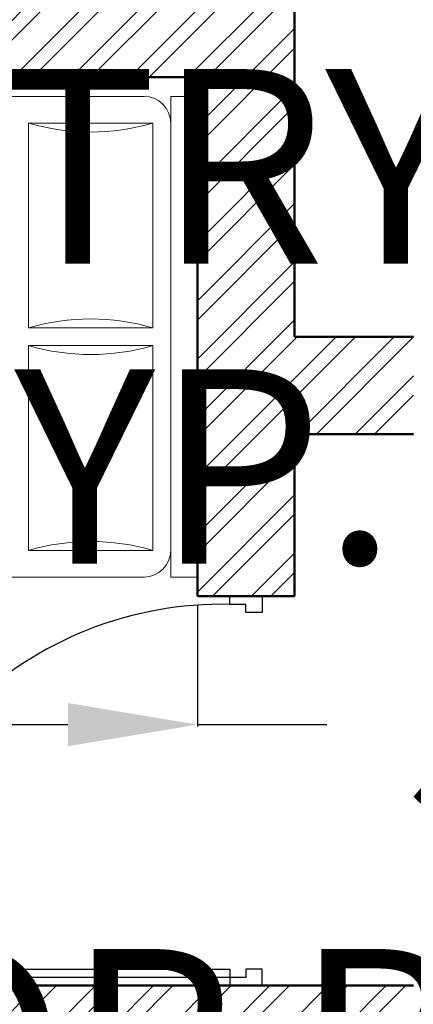
# Model space of a CAD drawing. Units: inches. Extents: x -90 to 536, y -553 to 299.
# Tile 9 of 27: x 155 to 191, y -430 to -339. Entities that reach past the tile are written whole.
import ezdxf

# ---------------------------------------------------------------- set-up
doc = ezdxf.new("R2010")
doc.units = ezdxf.units.IN
for name, color, linetype, lineweight in [('A-ANNO-DIMS', 2, 'Continuous', 18), ('A-DOOR', 4, 'Continuous', 25), ('A-WALL-PATT', 252, 'Continuous', 13), ('Furniture', 2, 'Continuous', 18), ('Outer Wall', 1, 'Continuous', 50)]:
    doc.layers.add(name, color=color, linetype=linetype, lineweight=lineweight)
doc.styles.get("Standard").update_dxf_attribs({"font": 'arial.ttf'})
doc.dimstyles.get("Standard").update_dxf_attribs({"dimtxt": 18, "dimasz": 12, "dimexe": 0.18, "dimexo": 0.0625, "dimgap": 0.09, "dimtad": 0, "dimtih": 1, "dimtoh": 1, "dimdec": 0, "dimzin": 0, "dimdsep": 46, "dimlunit": 3, "dimtxsty": 'Standard', "dimcen": 0.09, "dimadec": 0, "dimazin": 0, "dimtfac": 1, "dimtdec": 0, "dimtofl": 0, "dimtmove": 0, "dimatfit": 3, "dimfxl": 1, "dimtolj": 1, "dimtzin": 0, "dimarcsym": 0})

# ---------------------------------------------------------------- blocks, each defined once
blk = doc.blocks.new('A$C62731D1C')
for p, q in [((0.0963, 2.2932, 0.6857), (1.4679, 2.2932, 0.6857)), ((0.0963, 2.217, 0.6857), (0.0963, 2.2932, 0.6857)), ((1.4679, 2.217, 0.6857), (1.4679, 2.2932, 0.6857)), ((0.0963, 2.217, 0.6857), (1.4679, 2.217, 0.6857)), ((0.7567, 2.1662, 0.6857), (0.1725, 2.1662, 0.6857)), ((0.1725, 2.1662, 0.6857), (0.1725, 1.8106, 0.6857)), ((0.7567, 1.8106, 0.6857), (0.7567, 2.1662, 0.6857)), ((0.8075, 2.1662, 0.6857), (0.8075, 1.8106, 0.6857)), ((1.3917, 2.1662, 0.6857), (0.8075, 2.1662, 0.6857)), ((1.3917, 1.8106, 0.6857), (1.3917, 2.1662, 0.6857)), ((0.0963, 0.3882, 0.6857), (0.0963, 2.1408, 0.6857)), ((1.4679, 2.1408, 0.6857), (1.4679, 0.3882, 0.6857)), ((0.1725, 1.8106, 0.6857), (0.7567, 1.8106, 0.6857)), ((0.8075, 1.8106, 0.6857), (1.3917, 1.8106, 0.6857))]:
    blk.add_line(p, q)
for centre, radius, start, end in [((0.1725, 2.1408, 0.6857), 0.0762, 90, 180), ((1.3917, 2.1408, 0.6857), 0.0762, 0, 90), ((-0.4371, 1.9884, 0.6857), 0.635, 343.7398, 16.2602), ((1.3663, 1.9884, 0.6857), 0.635, 163.7398, 196.2602), ((0.1979, 1.9884, 0.6857), 0.635, 343.7398, 16.2602), ((2.0013, 1.9884, 0.6857), 0.635, 163.7398, 196.2602)]:
    blk.add_arc(centre, radius, start, end)
blk = doc.blocks.new('A$C0E6D7E3D')
blk.add_blockref('A$C62731D1C', (0, 0))
blk = doc.blocks.new('DOOR-36-B')
for points in [[(37.5, 36), (37.5, 34.5), (36, 34.5), (36, 35.25), (34.5, 35.25), (34.5, 36)], [(0, 0.75), (0, 1.5), (34.5, 1.5), (34.5, 0.75)], [(37.5, 0), (37.5, 1.5), (36, 1.5), (36, 0.75), (34.5, 0.75), (34.5, 0)]]:
    blk.add_lwpolyline(points, close=True)
blk.add_arc((33.758, 1.5), 33.758, 88.7408, 180)
blk = doc.blocks.new('*D27')
at = {"layer": 'A-ANNO-DIMS', "color": 0, "lineweight": -2, "transparency": 16777216}
for p, q in [((49.132, -428.616), (49.132, -434.359)), ((86.632, -428.616), (86.632, -434.359)), ((61.132, -434.179), (74.632, -434.179)), ((86.632, -434.179), (98.632, -434.179))]:
    blk.add_line(p, q, dxfattribs=at)
at = {"layer": 'A-ANNO-DIMS', "color": 0, "transparency": 16777216}
for points in [[(61.132, -432.179), (61.132, -436.179), (49.132, -434.179)], [(74.632, -432.179), (74.632, -436.179), (86.632, -434.179)]]:
    blk.add_solid(points, dxfattribs=at)
at = {"layer": 'Defpoints', "color": 0, "transparency": 16777216}
for p in [(49.132, -428.554), (86.632, -428.554), (86.632, -434.179)]:
    blk.add_point(p, dxfattribs=at)
at = {"layer": 'A-ANNO-DIMS', "color": 0, "transparency": 16777216, "insert": (195.174, -434.179), "char_height": 18, "attachment_point": 5}
blk.add_mtext('\\A1;DOOR B 38 TYP.', dxfattribs=at)
blk = doc.blocks.new('*D28')
at = {"layer": 'A-ANNO-DIMS', "color": 0, "lineweight": -2, "transparency": 16777216}
for p, q in [((92.257, -392.554), (92.257, -380.554)), ((92.257, -380.554), (104.257, -380.554)), ((86.694, -392.554), (92.437, -392.554)), ((92.257, -416.554), (92.257, -404.554)), ((86.694, -428.554), (92.437, -428.554))]:
    blk.add_line(p, q, dxfattribs=at)
at = {"layer": 'A-ANNO-DIMS', "color": 0, "transparency": 16777216}
for points in [[(90.257, -404.554), (94.257, -404.554), (92.257, -392.554)], [(90.257, -416.554), (94.257, -416.554), (92.257, -428.554)]]:
    blk.add_solid(points, dxfattribs=at)
at = {"layer": 'Defpoints', "color": 0, "transparency": 16777216}
for p in [(86.632, -392.554), (92.257, -392.554), (86.632, -428.554)]:
    blk.add_point(p, dxfattribs=at)
at = {"layer": 'A-ANNO-DIMS', "color": 0, "transparency": 16777216, "insert": (148.15, -380.554), "char_height": 18, "attachment_point": 5}
blk.add_mtext('\\A1;36 TYP.', dxfattribs=at)
blk = doc.blocks.new('*D35')
at = {"layer": 'A-ANNO-DIMS', "color": 0, "lineweight": -2, "transparency": 16777216}
for p, q in [((233.194, -331.054), (239.837, -331.054)), ((239.657, -343.054), (239.657, -343.401)), ((239.657, -362.554), (239.657, -362.207)), ((233.194, -374.554), (239.837, -374.554))]:
    blk.add_line(p, q, dxfattribs=at)
at = {"layer": 'A-ANNO-DIMS', "color": 0, "transparency": 16777216}
for points in [[(237.657, -343.054), (241.657, -343.054), (239.657, -331.054)], [(237.657, -362.554), (241.657, -362.554), (239.657, -374.554)]]:
    blk.add_solid(points, dxfattribs=at)
at = {"layer": 'Defpoints', "color": 0, "transparency": 16777216}
for p in [(233.132, -331.054), (239.657, -331.054), (233.132, -374.554)]:
    blk.add_point(p, dxfattribs=at)
at = {"layer": 'A-ANNO-DIMS', "color": 0, "transparency": 16777216, "insert": (239.657, -352.804), "char_height": 18, "attachment_point": 5}
blk.add_mtext('\\A1;ENTRY DOOR 44 TYP.', dxfattribs=at)
blk = doc.blocks.new('*D51')
at = {"layer": 'A-ANNO-DIMS', "color": 0, "lineweight": -2, "transparency": 16777216}
for p, q in [((96.806, -393.34), (96.806, -404.606)), ((171.132, -393.34), (171.132, -404.606)), ((108.806, -404.426), (159.132, -404.426)), ((171.132, -404.426), (183.132, -404.426))]:
    blk.add_line(p, q, dxfattribs=at)
at = {"layer": 'A-ANNO-DIMS', "color": 0, "transparency": 16777216}
for points in [[(108.806, -402.426), (108.806, -406.426), (96.806, -404.426)], [(159.132, -402.426), (159.132, -406.426), (171.132, -404.426)]]:
    blk.add_solid(points, dxfattribs=at)
at = {"layer": 'Defpoints', "color": 0, "transparency": 16777216}
for p in [(96.806, -393.277), (171.132, -393.277), (171.132, -404.426)]:
    blk.add_point(p, dxfattribs=at)
at = {"layer": 'A-ANNO-DIMS', "color": 0, "transparency": 16777216, "insert": (274.99, -404.426), "char_height": 18, "attachment_point": 5}
blk.add_mtext('\\A1;SINGLE BED 74', dxfattribs=at)

msp = doc.modelspace()

# ---------------------------------------------------------------- hatches: boundary and pattern name
at = {"layer": 'A-WALL-PATT'}
h = msp.add_hatch(dxfattribs=at)
h.set_pattern_fill('ANSI32', color=256, scale=0.4)
h.set_pattern_definition([(45, (-88.8105, -603.6155), (-2.694077, 2.694077), []), (45, (-87.0145, -603.6155), (-2.694077, 2.694077), [])])
h.paths.add_polyline_path([(285.1317, 246.4462), (131.1317, 246.4462), (131.1317, 237.4462), (285.1317, 237.4462)])
h.paths.add_polyline_path([(122.1317, 237.4462), (113.1317, 237.4462), (113.1317, 152.4462), (122.1317, 152.4462), (122.1317, 166.4704)])
h.paths.add_polyline_path([(303.1317, 237.4462), (294.1317, 237.4462), (294.1317, 152.4462), (303.1317, 152.4462)])
h.paths.add_polyline_path([(47.1317, 91.9277), (38.1317, 91.9277), (38.1317, -6.5538), (77.1317, -6.5538), (77.1317, 2.4462), (70.5655, 2.4462), (47.1317, 2.4462)])
h.paths.add_polyline_path([(83.052, -61.5538), (47.1317, -61.5538), (47.1317, -24.5538), (38.1317, -24.5538), (38.1317, -70.5538), (74.052, -70.5538), (74.052, -223.5538), (38.1317, -223.5538), (38.1317, -503.5538), (92.1317, -503.5538), (92.1317, -437.5538), (191.1317, -437.5538), (191.1317, -428.5538), (83.1317, -428.5538), (83.1317, -494.5538), (47.1317, -494.5538), (47.1317, -232.5538), (83.052, -232.5538), (83.052, -70.5538)])
h.paths.add_polyline_path([(407.1317, -63.5538), (381.1317, -63.5538), (381.1317, 91.9277), (372.1317, 91.9277), (372.1317, 32.8805), (372.1317, -63.5538), (306.5745, -63.5538), (237.1317, -63.5538), (237.1317, -38.5538), (233.1317, -38.5538), (233.1317, -71.5538), (398.1317, -71.5538), (398.1317, -152.5538), (233.1317, -152.5538), (233.1317, -161.5538), (398.1317, -161.5538), (398.1317, -368.5538), (233.1317, -368.5538), (233.1317, -377.5538), (407.1317, -377.5538), (407.1317, -161.5538)])
h.paths.add_polyline_path([(261.1317, -422.5538), (252.1317, -422.5538), (252.1317, -428.5538), (233.1317, -428.5538), (233.1317, -437.5538), (261.1317, -437.5538)])
h.paths.add_polyline_path([(191.1317, -368.5538), (180.1317, -368.5538), (180.1317, -335.5538), (131.5919, -335.5538), (131.5919, -344.5538), (171.1317, -344.5538), (171.1317, -392.5538), (180.1317, -392.5538), (180.1317, -377.5538), (191.1317, -377.5538)], flags=17)
h.paths.add_polyline_path([(180.1317, -223.5538), (152.1317, -223.5538), (152.1317, -227.5538), (176.1317, -227.5538), (176.1317, -335.5538), (180.1317, -335.5538)], flags=17)
h.paths.add_polyline_path([(131.5919, -335.5538), (83.1317, -335.5538), (83.1317, -339.5538), (83.1317, -392.5538), (87.1317, -392.5538), (87.1317, -339.5538), (131.5919, -339.5538)], flags=17)
h.paths.add_polyline_path([(197.1317, 2.4462), (77.1317, 2.4462), (77.1317, -1.5538), (113.1317, -1.5538), (113.1317, -71.5538), (181.1317, -71.5538), (181.1317, -67.5538), (117.1317, -67.5538), (117.1317, -1.5538), (177.1317, -1.5538), (177.1317, -37.5538), (181.1317, -37.5538), (181.1317, -1.5538), (197.1317, -1.5538)])
h.paths.add_polyline_path([(173.1317, 138.4462), (122.1317, 138.4462), (122.1317, 134.4462), (173.1317, 134.4462)])
h.paths.add_polyline_path([(213.1317, 237.4462), (209.1317, 237.4462), (209.1317, 134.4462), (233.1317, 134.4462), (233.1317, 68.8889), (233.1317, -2.5538), (237.1317, -2.5538), (237.1317, 134.4462), (258.1317, 134.4462), (258.1317, 138.4462), (213.1317, 138.4462)])

# ---------------------------------------------------------------- linework, layer by layer
at = {"layer": 'Outer Wall'}
for p, q in [((180.1317, -368.5538), (180.1317, -335.5538)), ((131.5919, -344.5538), (171.1317, -344.5538)), ((171.1317, -392.5538), (171.1317, -344.5538)), ((191.1317, -368.5538), (180.1317, -368.5538)), ((180.1317, -392.5538), (180.1317, -377.5538)), ((191.1317, -377.5538), (180.1317, -377.5538)), ((180.1317, -392.5538), (171.1317, -392.5538)), ((191.1317, -428.5538), (83.1317, -428.5538))]:
    msp.add_line(p, q, dxfattribs=at)

# ---------------------------------------------------------------- block references
at = {"layer": 'A-DOOR'}
msp.add_blockref('DOOR-36-B', (139.6317, -428.5538), dxfattribs=at)
at = {"layer": 'Furniture', "xscale": 32.41097235378273, "yscale": 32.41097235378273, "zscale": 32.41097235378273, "rotation": 270}
msp.add_blockref('A$C0E6D7E3D', (96.8056, -343.2061, -22.2246), dxfattribs=at)

# ---------------------------------------------------------------- dimensions: what is measured, and where the dimension line sits
at = {"layer": 'A-ANNO-DIMS'}
for base, p1, p2, text, picture, middle in [((239.6567404714, -331.0537825705), (233.1317404714, -374.5537825705), (233.1317404714, -331.0537825705), 'ENTRY DOOR <> TYP.', '*D35', (239.6567404714, -352.8037825705)), ((92.2567, -392.5538), (86.6317, -428.5538), (86.6317, -392.5538), '<> TYP.', '*D28', (148.1496, -380.5538))]:
    dim = msp.add_linear_dim(base=base, p1=p1, p2=p2, angle=90, text=text, dimstyle='Standard', override={"dimdec": 0, "dimlfac": 1, "dimrnd": 0, "dimzin": 0, "dimdsep": 46, "dimlunit": 2}, dxfattribs=at)
    dim.commit()
    dim.dimension.update_dxf_attribs({"geometry": picture, "text_midpoint": middle})
for base, p1, p2, text, picture, middle in [((171.1317, -404.4263), (96.8056, -393.2773), (171.1317, -393.2773), 'SINGLE BED <>', '*D51', (274.9898, -404.4263)), ((86.6317404714, -434.1787825705), (49.1317404714, -428.5537825705), (86.6317404714, -428.5537825705), 'DOOR B <> TYP.', '*D27', (195.1739914946, -434.1787825705))]:
    dim = msp.add_linear_dim(base=base, p1=p1, p2=p2, text=text, dimstyle='Standard', override={"dimdec": 0, "dimlfac": 1, "dimrnd": 0, "dimzin": 0, "dimdsep": 46, "dimlunit": 2}, dxfattribs=at)
    dim.commit()
    dim.dimension.update_dxf_attribs({"geometry": picture, "text_midpoint": middle})

doc.saveas('drawing.dxf')
